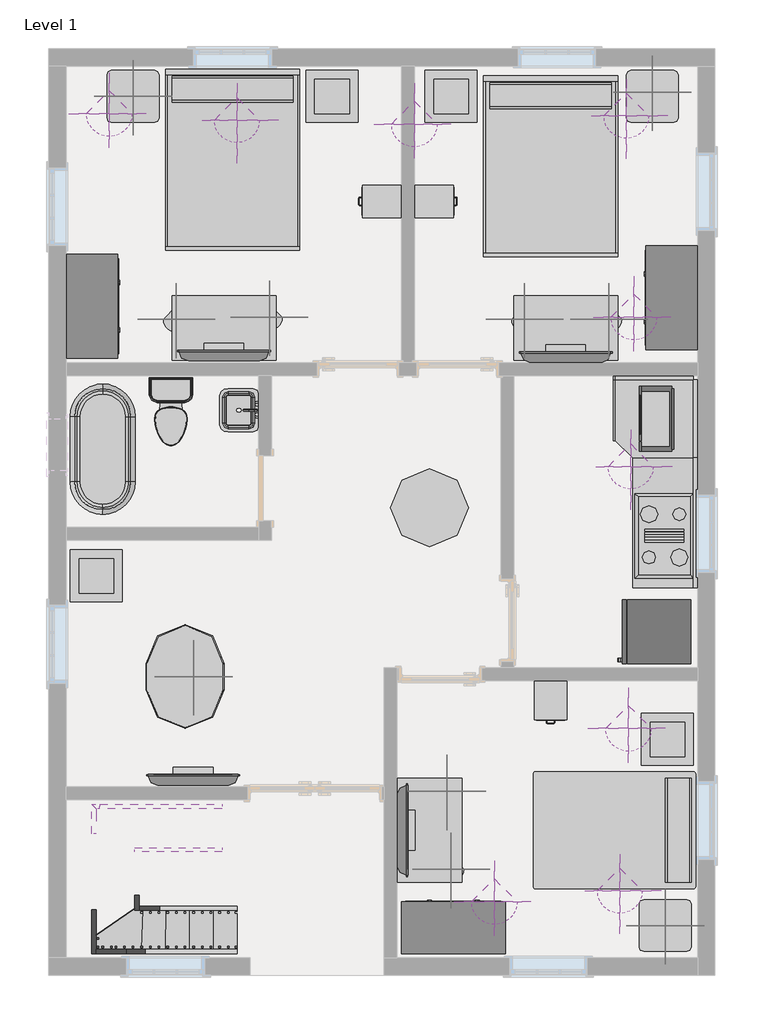
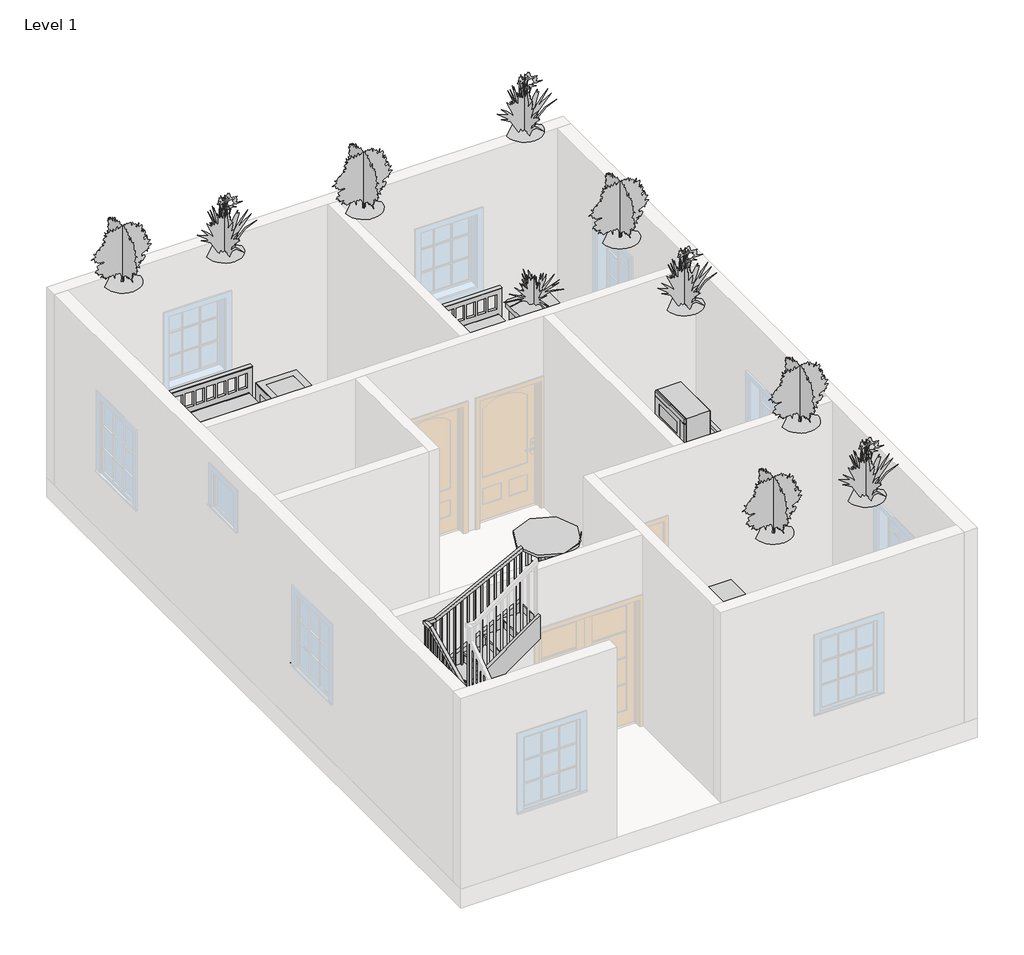
# One storey, part 2 of 2: 26 furniture elements, 19 geographic elements, 9 members, 4 flow terminals, 3 proxies, 1 railing, 1 stair flight.
"""IFC4 building model written with IfcOpenShell, lengths in millimetres."""

from ifc_helpers import new_model, si_unit, frame, origin, place, context, project, spatial, polyline, outline, extrude, faceted_brep, transform, mapped, element, save
from components import proxy_bb1e6e30, proxy_8a8d5ab2, proxy_a13a33b2, flow_terminal_accce45a, flow_terminal_62a433f7, toilet_domestic_3d_toilet_domestic_3d_f7549cf7, toilet_domestic_3d_toilet_domestic_3d_183bbd19, flow_terminal_b374fae2, furniture_35c09872, furniture_0253826f, furniture_bb55ed6b, furniture_9fa109b2, furniture_7a3aaa4f, furniture_b5c51a22, furniture_be1c6672, furniture_905aceb5, furniture_31d08a24, furniture_3f969c1c, furniture_f408c91c, rpc_plant_tropical_55f6ff97, rpc_plant_tropical_agave_1_5_93a2a214, rpc_plant_tropical_jungle_flame_3_9c4808c2, stair_flight_132ddc74

model = new_model("IFC4")

# Units and contexts
model_context = context("Model", 3, world=origin())
ifc_project = project(units=[si_unit("LENGTHUNIT", "METRE", prefix="MILLI")], contexts=[model_context])

# Site, building, storey
site = spatial("IfcSite", under=ifc_project)
building = spatial("IfcBuilding", under=site)
storey = spatial("IfcBuildingStorey", under=building, Name="Level 1", Elevation=0.0)

# Proxies
placement = place(None, origin())
proxy_shape = proxy_bb1e6e30(model_context)
element("IfcBuildingElementProxy", 1, Name="Cook Top-4 Unit : 36\" x 20\"", ObjectType="Cook Top-4 Unit : 36\" x 20\"", at=placement, inside=storey, context=model_context, shape_type="MappedRepresentation", body=[
    mapped(proxy_shape, transform((-5830.7047602, 8433.499435, 0.0), x_axis=(0.0, 1.0000000000000002, 0.0), y_axis=(-1.0000000000000002, 0.0, 0.0), z_axis=(0.0, 0.0, 1.0))),
])
proxy_2_shape = proxy_8a8d5ab2(model_context)
element("IfcBuildingElementProxy", 2, Name="Microwave : 30\" x 16\" x 18\"", ObjectType="Microwave : 30\" x 16\" x 18\"", at=placement, inside=storey, context=model_context, shape_type="MappedRepresentation", body=[
    mapped(proxy_2_shape, transform((-5566.5242544, 10305.3923123, 0.0), x_axis=(0.0, -1.0000000000000004, 0.0), y_axis=(1.0000000000000004, 0.0, 0.0), z_axis=(0.0, 0.0, 1.0))),
])
proxy_3_shape = proxy_a13a33b2(model_context)
element("IfcBuildingElementProxy", 3, Name="Refrigerator : 30\" x 32\" RH", ObjectType="Refrigerator : 30\" x 32\" RH", at=placement, inside=storey, context=model_context, shape_type="MappedRepresentation", body=[
    mapped(proxy_3_shape, transform((-5905.3172602, 7308.3504635, 0.0), x_axis=(0.0, -1.0000000000000007, 0.0), y_axis=(1.0000000000000007, 0.0, 0.0), z_axis=(0.0, 0.0, 1.0))),
])

# Flow terminals
flow_terminal_shape = flow_terminal_accce45a(model_context)
element("IfcFlowTerminal", 4, ObjectType="Floor Drain - Round : 5\" Strainer - 2\" Drain", at=placement, inside=storey, context=model_context, shape_type="MappedRepresentation", body=[
    mapped(flow_terminal_shape, transform((-11812.4047602, 8865.299435, 0.0), x_axis=(1.0, 0.0, 0.0), y_axis=(0.0, 1.0, 0.0), z_axis=(0.0, 0.0, 1.0))),
])
flow_terminal_2_shape = flow_terminal_62a433f7(model_context)
element("IfcFlowTerminal", 5, ObjectType="Sink Vanity-Square : 20\" x 18\"", at=placement, inside=storey, context=model_context, shape_type="MappedRepresentation", body=[
    mapped(flow_terminal_2_shape, transform((-10773.3501613, 9922.3886756, 0.0), x_axis=(0.0, -1.0000000000000002, 0.0), y_axis=(1.0000000000000002, 0.0, 0.0), z_axis=(0.0, 0.0, 1.0))),
])
toilet_domestic_3d_toilet_domestic_3d_shape = toilet_domestic_3d_toilet_domestic_3d_f7549cf7(model_context)
toilet_domestic_3d_toilet_domestic_3d_2_shape = toilet_domestic_3d_toilet_domestic_3d_183bbd19(model_context)
element("IfcFlowTerminal", 6, ObjectType="Toilet-Domestic-3D : Toilet-Domestic-3D", at=placement, inside=storey, context=model_context, shape_type="MappedRepresentation", body=[
    mapped(toilet_domestic_3d_toilet_domestic_3d_shape, transform((-11621.9047602, 9793.0034076, 0.0), x_axis=(1.0, 0.0, 0.0), y_axis=(0.0, 1.0, 0.0), z_axis=(0.0, 0.0, 1.0))),
    mapped(toilet_domestic_3d_toilet_domestic_3d_2_shape, transform((-11621.9047602, 9793.0034076, 0.0), x_axis=(1.0, 0.0, 0.0), y_axis=(0.0, 1.0, 0.0), z_axis=(0.0, 0.0, 1.0))),
])
flow_terminal_3_shape = flow_terminal_b374fae2(model_context)
element("IfcFlowTerminal", 7, ObjectType="Tub-Free Standing-3D : 30\" x 60\"", at=placement, inside=storey, context=model_context, shape_type="MappedRepresentation", body=[
    mapped(flow_terminal_3_shape, transform((-12422.0047602, 9449.499435, 0.0), x_axis=(1.0, 0.0, 0.0), y_axis=(0.0, 1.0, 0.0), z_axis=(0.0, 0.0, 1.0))),
])

# Furniture
furniture_shape = furniture_35c09872(model_context)
element("IfcFurniture", 8, ObjectType="Bed-Shaker : Queen 62\" x 83\"", at=placement, inside=storey, context=model_context, shape_type="MappedRepresentation", body=[
    mapped(furniture_shape, transform((-10878.9547602, 13894.499435, 0.0), x_axis=(1.0, 0.0, 0.0), y_axis=(0.0, 1.0, 0.0), z_axis=(0.0, 0.0, 1.0))),
])
element("IfcFurniture", 9, ObjectType="Bed-Shaker : Queen 62\" x 83\"", at=placement, inside=storey, context=model_context, shape_type="MappedRepresentation", body=[
    mapped(furniture_shape, transform((-7145.1547602, 13818.299435, 0.0), x_axis=(1.0, 0.0, 0.0), y_axis=(0.0, 1.0, 0.0), z_axis=(0.0, 0.0, 1.0))),
])
furniture_2_shape = furniture_0253826f(model_context)
element("IfcFurniture", 10, ObjectType="Bed-Standard.0001 : Double 54\" x 75\"", at=placement, inside=storey, context=model_context, shape_type="MappedRepresentation", body=[
    mapped(furniture_2_shape, transform((-6369.3096782, 5250.5879596, 0.0), x_axis=(0.0, -1.0000000000000002, 0.0), y_axis=(1.0000000000000002, 0.0, 0.0), z_axis=(0.0, 0.0, 1.0))),
])
furniture_3_shape = furniture_bb55ed6b(model_context)
element("IfcFurniture", 11, ObjectType="Cabinet-File 2 Drawer : 15\" x 18\"", at=placement, inside=storey, context=model_context, shape_type="MappedRepresentation", body=[
    mapped(furniture_3_shape, transform((-9003.2704601, 12229.9029879, 0.0), x_axis=(0.0, -1.0000000000000002, 0.0), y_axis=(1.0000000000000002, 0.0, 0.0), z_axis=(0.0, 0.0, 1.0))),
])
element("IfcFurniture", 12, ObjectType="Cabinet-File 2 Drawer : 15\" x 18\"", at=placement, inside=storey, context=model_context, shape_type="MappedRepresentation", body=[
    mapped(furniture_3_shape, transform((-8677.9390603, 12485.695882, 0.0), x_axis=(0.0, 1.0, 0.0), y_axis=(-1.0, 0.0, 0.0), z_axis=(0.0, 0.0, 1.0))),
])
element("IfcFurniture", 13, ObjectType="Cabinet-File 2 Drawer : 15\" x 18\"", at=placement, inside=storey, context=model_context, shape_type="MappedRepresentation", body=[
    mapped(furniture_3_shape, transform((-7036.2699762, 6645.2337351, 0.0), x_axis=(1.0, 0.0, 0.0), y_axis=(0.0, 1.0, 0.0), z_axis=(0.0, 0.0, 1.0))),
])
furniture_4_shape = furniture_9fa109b2(model_context)
element("IfcFurniture", 14, ObjectType="Dresser : 48\" x 72\" x 24\"", at=placement, inside=storey, context=model_context, shape_type="MappedRepresentation", body=[
    mapped(furniture_4_shape, transform((-12912.1677143, 11395.0926948, 0.0), x_axis=(0.0, 1.0, 0.0), y_axis=(-1.0, 0.0, 0.0), z_axis=(0.0, 0.0, 1.0))),
])
element("IfcFurniture", 15, ObjectType="Dresser : 48\" x 72\" x 24\"", at=placement, inside=storey, context=model_context, shape_type="MappedRepresentation", body=[
    mapped(furniture_4_shape, transform((-5378.6418061, 10958.3061751, 0.0), x_axis=(0.0, -1.0000000000000004, 0.0), y_axis=(1.0000000000000004, 0.0, 0.0), z_axis=(0.0, 0.0, 1.0))),
])
element("IfcFurniture", 16, ObjectType="Dresser : 48\" x 72\" x 24\"", at=placement, inside=storey, context=model_context, shape_type="MappedRepresentation", body=[
    mapped(furniture_4_shape, transform((-8576.3980201, 3472.9364809, 0.0), x_axis=(-1.0000000000000004, 0.0, 0.0), y_axis=(0.0, -1.0000000000000004, 0.0), z_axis=(0.0, 0.0, 1.0))),
])
furniture_5_shape = furniture_7a3aaa4f(model_context)
element("IfcFurniture", 17, ObjectType="TV - Flat Screen : 42\"", at=placement, inside=storey, context=model_context, shape_type="MappedRepresentation", body=[
    mapped(furniture_5_shape, transform((-11003.5492744, 10543.0880586, 1041.4), x_axis=(-1.0000000000000004, 0.0, 0.0), y_axis=(0.0, -1.0000000000000004, 0.0), z_axis=(0.0, 0.0, 1.0))),
])
element("IfcFurniture", 18, ObjectType="TV - Flat Screen : 42\"", at=placement, inside=storey, context=model_context, shape_type="MappedRepresentation", body=[
    mapped(furniture_5_shape, transform((-6990.3492744, 10524.0380586, 1041.4), x_axis=(-1.0000000000000004, 0.0, 0.0), y_axis=(0.0, -1.0000000000000004, 0.0), z_axis=(0.0, 0.0, 1.0))),
])
element("IfcFurniture", 19, ObjectType="TV - Flat Screen : 42\"", at=placement, inside=storey, context=model_context, shape_type="MappedRepresentation", body=[
    mapped(furniture_5_shape, transform((-8909.0661366, 4983.0439491, 1041.4), x_axis=(0.0, 1.0000000000000002, 0.0), y_axis=(-1.0000000000000002, 0.0, 0.0), z_axis=(0.0, 0.0, 1.0))),
])
element("IfcFurniture", 20, ObjectType="TV - Flat Screen : 42\"", at=placement, inside=storey, context=model_context, shape_type="MappedRepresentation", body=[
    mapped(furniture_5_shape, transform((-11365.4992744, 5564.6880586, 990.6), x_axis=(-1.0, 0.0, 0.0), y_axis=(0.0, -1.0, 0.0), z_axis=(0.0, 0.0, 1.0))),
])
furniture_6_shape = furniture_b5c51a22(model_context)
element("IfcFurniture", 21, ObjectType="Table-Coffee : 24\" x 24\" x 24\"", at=placement, inside=storey, context=model_context, shape_type="MappedRepresentation", body=[
    mapped(furniture_6_shape, transform((-9747.8705269, 13494.4883572, 0.0), x_axis=(1.0, 0.0, 0.0), y_axis=(0.0, 1.0, 0.0), z_axis=(0.0, 0.0, 1.0))),
])
element("IfcFurniture", 22, ObjectType="Table-Coffee : 24\" x 24\" x 24\"", at=placement, inside=storey, context=model_context, shape_type="MappedRepresentation", body=[
    mapped(furniture_6_shape, transform((-8350.8705269, 13494.4883572, 0.0), x_axis=(1.0, 0.0, 0.0), y_axis=(0.0, 1.0, 0.0), z_axis=(0.0, 0.0, 1.0))),
])
element("IfcFurniture", 23, ObjectType="Table-Coffee : 24\" x 24\" x 24\"", at=placement, inside=storey, context=model_context, shape_type="MappedRepresentation", body=[
    mapped(furniture_6_shape, transform((-12516.4705269, 7868.3883572, 0.0), x_axis=(1.0, 0.0, 0.0), y_axis=(0.0, 1.0, 0.0), z_axis=(0.0, 0.0, 1.0))),
])
element("IfcFurniture", 24, ObjectType="Table-Coffee : 24\" x 24\" x 24\"", at=placement, inside=storey, context=model_context, shape_type="MappedRepresentation", body=[
    mapped(furniture_6_shape, transform((-5810.8705269, 5950.6883572, 0.0), x_axis=(1.0, 0.0, 0.0), y_axis=(0.0, 1.0, 0.0), z_axis=(0.0, 0.0, 1.0))),
])
furniture_7_shape = furniture_be1c6672(model_context)
element("IfcFurniture", 25, ObjectType="Table-Dining Oval : 36\" x 48\"", at=placement, inside=storey, context=model_context, shape_type="MappedRepresentation", body=[
    mapped(furniture_7_shape, transform((-11814.9031209, 7184.3191071, 0.0), x_axis=(0.0, 1.0000000000000002, 0.0), y_axis=(-1.0000000000000002, 0.0, 0.0), z_axis=(0.0, 0.0, 1.0))),
])
furniture_8_shape = furniture_905aceb5(model_context)
element("IfcFurniture", 26, ObjectType="Table-Dining Round w Chairs : 36\" Diameter", at=placement, inside=storey, context=model_context, shape_type="MappedRepresentation", body=[
    mapped(furniture_8_shape, transform((-8690.2867274, 8948.5781235, 0.0), x_axis=(1.0, 0.0, 0.0), y_axis=(0.0, 1.0, 0.0), z_axis=(0.0, 0.0, 1.0))),
])
furniture_9_shape = furniture_31d08a24(model_context)
element("IfcFurniture", 27, ObjectType="Table-End : 24\" x 24\"", at=placement, inside=storey, context=model_context, shape_type="MappedRepresentation", body=[
    mapped(furniture_9_shape, transform((-12374.9383905, 13437.299435, 0.0), x_axis=(1.0, 0.0, 0.0), y_axis=(0.0, 1.0, 0.0), z_axis=(0.0, 0.0, 1.0))),
])
element("IfcFurniture", 28, ObjectType="Table-End : 24\" x 24\"", at=placement, inside=storey, context=model_context, shape_type="MappedRepresentation", body=[
    mapped(furniture_9_shape, transform((-6278.9383905, 13437.299435, 0.0), x_axis=(1.0, 0.0, 0.0), y_axis=(0.0, 1.0, 0.0), z_axis=(0.0, 0.0, 1.0))),
])
element("IfcFurniture", 29, ObjectType="Table-End : 24\" x 24\"", at=placement, inside=storey, context=model_context, shape_type="MappedRepresentation", body=[
    mapped(furniture_9_shape, transform((-6126.5383905, 3709.099435, 0.0), x_axis=(1.0, 0.0, 0.0), y_axis=(0.0, 1.0, 0.0), z_axis=(0.0, 0.0, 1.0))),
])
furniture_10_shape = furniture_3f969c1c(model_context)
element("IfcFurniture", 30, ObjectType="Table-Rectangular : 72\" x 30\"", at=placement, inside=storey, context=model_context, shape_type="MappedRepresentation", body=[
    mapped(furniture_10_shape, transform((-10999.6047602, 10871.899435, 0.0), x_axis=(1.0, 0.0, 0.0), y_axis=(0.0, 1.0, 0.0), z_axis=(0.0, 0.0, 1.0))),
])
element("IfcFurniture", 31, ObjectType="Table-Rectangular : 72\" x 30\"", at=placement, inside=storey, context=model_context, shape_type="MappedRepresentation", body=[
    mapped(furniture_10_shape, transform((-6986.4047602, 10871.899435, 0.0), x_axis=(1.0, 0.0, 0.0), y_axis=(0.0, 1.0, 0.0), z_axis=(0.0, 0.0, 1.0))),
])
element("IfcFurniture", 32, ObjectType="Table-Rectangular : 72\" x 30\"", at=placement, inside=storey, context=model_context, shape_type="MappedRepresentation", body=[
    mapped(furniture_10_shape, transform((-8586.6047602, 4979.099435, 0.0), x_axis=(0.0, 1.0000000000000002, 0.0), y_axis=(-1.0000000000000002, 0.0, 0.0), z_axis=(0.0, 0.0, 1.0))),
])
furniture_11_shape = furniture_f408c91c(model_context)
element("IfcFurniture", 33, ObjectType="Work Station Cubicle : 96\" x 96\"", at=placement, inside=storey, context=model_context, shape_type="MappedRepresentation", body=[
    mapped(furniture_11_shape, transform((-4941.9817526, 10181.3676828, 0.0), x_axis=(0.0, -1.0000000000000004, 0.0), y_axis=(1.0000000000000004, 0.0, 0.0), z_axis=(0.0, 0.0, 1.0))),
])

# Geographic elements
rpc_plant_tropical_shape = rpc_plant_tropical_55f6ff97(model_context)
element("IfcGeographicElement", 34, ObjectType="RPC Plant - Tropical", at=placement, inside=storey, context=model_context, shape_type="MappedRepresentation", body=[
    mapped(rpc_plant_tropical_shape, transform((-6275.2047602, 13361.099435, 3657.6), x_axis=(1.0, 0.0, 0.0), y_axis=(0.0, 1.0, 0.0), z_axis=(0.0, 0.0, 1.0))),
])
element("IfcGeographicElement", 35, ObjectType="RPC Plant - Tropical", at=placement, inside=storey, context=model_context, shape_type="MappedRepresentation", body=[
    mapped(rpc_plant_tropical_shape, transform((-10847.2047602, 13310.299435, 3352.8), x_axis=(1.0, 0.0, 0.0), y_axis=(0.0, 1.0, 0.0), z_axis=(0.0, 0.0, 1.0))),
])
element("IfcGeographicElement", 36, ObjectType="RPC Plant - Tropical", at=placement, inside=storey, context=model_context, shape_type="MappedRepresentation", body=[
    mapped(rpc_plant_tropical_shape, transform((-6351.4047602, 4267.899435, 3352.8), x_axis=(1.0, 0.0, 0.0), y_axis=(0.0, 1.0, 0.0), z_axis=(0.0, 0.0, 1.0))),
])
element("IfcGeographicElement", 37, ObjectType="RPC Plant - Tropical", at=placement, inside=storey, context=model_context, shape_type="MappedRepresentation", body=[
    mapped(rpc_plant_tropical_shape, transform((-6224.4047602, 9246.299435, 3352.8), x_axis=(1.0, 0.0, 0.0), y_axis=(0.0, 1.0, 0.0), z_axis=(0.0, 0.0, 1.0))),
])
rpc_plant_tropical_agave_1_5_shape = rpc_plant_tropical_agave_1_5_93a2a214(model_context)
element("IfcGeographicElement", 38, ObjectType="RPC Plant - Tropical : Agave - 1.5'", at=placement, inside=storey, context=model_context, shape_type="MappedRepresentation", body=[
    mapped(rpc_plant_tropical_agave_1_5_shape, transform((-12066.4047602, 13589.699435, 609.6), x_axis=(1.0, 0.0, 0.0), y_axis=(0.0, 1.0, 0.0), z_axis=(0.0, 0.0, 1.0))),
])
element("IfcGeographicElement", 39, ObjectType="RPC Plant - Tropical : Agave - 1.5'", at=placement, inside=storey, context=model_context, shape_type="MappedRepresentation", body=[
    mapped(rpc_plant_tropical_agave_1_5_shape, transform((-11558.4047602, 10973.499435, 660.4), x_axis=(1.0, 0.0, 0.0), y_axis=(0.0, 1.0, 0.0), z_axis=(0.0, 0.0, 1.0))),
])
element("IfcGeographicElement", 40, ObjectType="RPC Plant - Tropical : Agave - 1.5'", at=placement, inside=storey, context=model_context, shape_type="MappedRepresentation", body=[
    mapped(rpc_plant_tropical_agave_1_5_shape, transform((-10466.2047602, 10998.899435, 660.4), x_axis=(1.0, 0.0, 0.0), y_axis=(0.0, 1.0, 0.0), z_axis=(0.0, 0.0, 1.0))),
])
element("IfcGeographicElement", 41, ObjectType="RPC Plant - Tropical : Agave - 1.5'", at=placement, inside=storey, context=model_context, shape_type="MappedRepresentation", body=[
    mapped(rpc_plant_tropical_agave_1_5_shape, transform((-5970.4047602, 13640.499435, 609.6), x_axis=(1.0, 0.0, 0.0), y_axis=(0.0, 1.0, 0.0), z_axis=(0.0, 0.0, 1.0))),
])
element("IfcGeographicElement", 42, ObjectType="RPC Plant - Tropical : Agave - 1.5'", at=placement, inside=storey, context=model_context, shape_type="MappedRepresentation", body=[
    mapped(rpc_plant_tropical_agave_1_5_shape, transform((-7469.0047602, 10973.499435, 660.4), x_axis=(1.0, 0.0, 0.0), y_axis=(0.0, 1.0, 0.0), z_axis=(0.0, 0.0, 1.0))),
])
element("IfcGeographicElement", 43, ObjectType="RPC Plant - Tropical : Agave - 1.5'", at=placement, inside=storey, context=model_context, shape_type="MappedRepresentation", body=[
    mapped(rpc_plant_tropical_agave_1_5_shape, transform((-6478.4047602, 10973.499435, 660.4), x_axis=(1.0, 0.0, 0.0), y_axis=(0.0, 1.0, 0.0), z_axis=(0.0, 0.0, 1.0))),
])
element("IfcGeographicElement", 44, ObjectType="RPC Plant - Tropical : Agave - 1.5'", at=placement, inside=storey, context=model_context, shape_type="MappedRepresentation", body=[
    mapped(rpc_plant_tropical_agave_1_5_shape, transform((-11355.2047602, 6782.499435, 736.6), x_axis=(1.0, 0.0, 0.0), y_axis=(0.0, 1.0, 0.0), z_axis=(0.0, 0.0, 1.0))),
])
element("IfcGeographicElement", 45, ObjectType="RPC Plant - Tropical : Agave - 1.5'", at=placement, inside=storey, context=model_context, shape_type="MappedRepresentation", body=[
    mapped(rpc_plant_tropical_agave_1_5_shape, transform((-5818.0047602, 3861.499435, 609.6), x_axis=(1.0, 0.0, 0.0), y_axis=(0.0, 1.0, 0.0), z_axis=(0.0, 0.0, 1.0))),
])
element("IfcGeographicElement", 46, ObjectType="RPC Plant - Tropical : Agave - 1.5'", at=placement, inside=storey, context=model_context, shape_type="MappedRepresentation", body=[
    mapped(rpc_plant_tropical_agave_1_5_shape, transform((-8383.4047602, 5436.299435, 660.4), x_axis=(1.0, 0.0, 0.0), y_axis=(0.0, 1.0, 0.0), z_axis=(0.0, 0.0, 1.0))),
])
element("IfcGeographicElement", 47, ObjectType="RPC Plant - Tropical : Agave - 1.5'", at=placement, inside=storey, context=model_context, shape_type="MappedRepresentation", body=[
    mapped(rpc_plant_tropical_agave_1_5_shape, transform((-8332.6047602, 4521.899435, 660.4), x_axis=(1.0, 0.0, 0.0), y_axis=(0.0, 1.0, 0.0), z_axis=(0.0, 0.0, 1.0))),
])
rpc_plant_tropical_jungle_flame_3_shape = rpc_plant_tropical_jungle_flame_3_9c4808c2(model_context)
element("IfcGeographicElement", 48, ObjectType="RPC Plant - Tropical : Jungle Flame - 3'", at=placement, inside=storey, context=model_context, shape_type="MappedRepresentation", body=[
    mapped(rpc_plant_tropical_jungle_flame_3_shape, transform((-8764.4047602, 13263.9821211, 3352.8), x_axis=(1.0, 0.0, 0.0), y_axis=(0.0, 1.0, 0.0), z_axis=(0.0, 0.0, 1.0))),
])
element("IfcGeographicElement", 49, ObjectType="RPC Plant - Tropical : Jungle Flame - 3'", at=placement, inside=storey, context=model_context, shape_type="MappedRepresentation", body=[
    mapped(rpc_plant_tropical_jungle_flame_3_shape, transform((-12345.8047602, 13386.499435, 3352.8), x_axis=(1.0, 0.0, 0.0), y_axis=(0.0, 1.0, 0.0), z_axis=(0.0, 0.0, 1.0))),
])
element("IfcGeographicElement", 50, ObjectType="RPC Plant - Tropical : Jungle Flame - 3'", at=placement, inside=storey, context=model_context, shape_type="MappedRepresentation", body=[
    mapped(rpc_plant_tropical_jungle_flame_3_shape, transform((-6186.3047602, 10998.899435, 3352.8), x_axis=(1.0, 0.0, 0.0), y_axis=(0.0, 1.0, 0.0), z_axis=(0.0, 0.0, 1.0))),
])
element("IfcGeographicElement", 51, ObjectType="RPC Plant - Tropical : Jungle Flame - 3'", at=placement, inside=storey, context=model_context, shape_type="MappedRepresentation", body=[
    mapped(rpc_plant_tropical_jungle_flame_3_shape, transform((-7824.6047602, 4140.899435, 3352.8), x_axis=(1.0, 0.0, 0.0), y_axis=(0.0, 1.0, 0.0), z_axis=(0.0, 0.0, 1.0))),
])
element("IfcGeographicElement", 52, ObjectType="RPC Plant - Tropical : Jungle Flame - 3'", at=placement, inside=storey, context=model_context, shape_type="MappedRepresentation", body=[
    mapped(rpc_plant_tropical_jungle_flame_3_shape, transform((-6249.8047602, 6172.899435, 3352.8), x_axis=(1.0, 0.0, 0.0), y_axis=(0.0, 1.0, 0.0), z_axis=(0.0, 0.0, 1.0))),
])

# Members
element("IfcMember", 53, ObjectType="Stringer - 2\" Width", at=placement, inside=storey, context=model_context, shape_type="SweptSolid", body=[
    extrude(outline(polyline([(196.4096939, -10847.2047602), (551.886059, -10847.2047602), (1331.4686735, -12146.2117977), (975.9923084, -12146.2117977), (196.4096939, -10847.2047602)])), frame((0.0, 3531.299435, 0.0), z_axis=(0.0, 1.0, 0.0), x_axis=(0.0, 0.0, 1.0)), (0.0, 0.0, 1.0), 50.8),
])
element("IfcMember", 54, ObjectType="Stringer - 2\" Width", at=placement, inside=storey, context=model_context, shape_type="SweptSolid", body=[
    extrude(outline(polyline([(-12146.2117977, 3582.099435), (-12146.2117977, 3531.299435), (-12501.9364521, 3531.299435), (-12501.9364521, 3582.099435), (-12146.2117977, 3582.099435)])), frame((0.0, 0.0, 975.9923084), z_axis=(0.0, 0.0, 1.0), x_axis=(1.0, 0.0, 0.0)), (0.0, 0.0, 1.0), 355.4763651),
])
element("IfcMember", 55, ObjectType="Stringer - 2\" Width", at=placement, inside=storey, context=model_context, shape_type="SweptSolid", body=[
    extrude(outline(polyline([(3531.299435, 1026.6686735), (3531.299435, 1306.8449342), (4939.7837414, 1989.5644288), (4939.7837414, 1634.0880637), (3686.6472991, 1026.6686735), (3531.299435, 1026.6686735)])), frame((-12552.7364521, 0.0, 0.0), z_axis=(1.0, 0.0, 0.0), x_axis=(0.0, 1.0, 0.0)), (0.0, 0.0, 1.0), 50.8),
])
element("IfcMember", 56, ObjectType="Stringer - 2\" Width", at=placement, inside=storey, context=model_context, shape_type="SweptSolid", body=[
    extrude(outline(polyline([(-12501.9364521, 4939.7837414), (-12552.7364521, 4939.7837414), (-12552.7364521, 5283.899435), (-12501.9364521, 5233.099435), (-12501.9364521, 4939.7837414)])), frame((0.0, 0.0, 1641.2436104), z_axis=(0.0, 0.0, 1.0), x_axis=(1.0, 0.0, 0.0)), (0.0, 0.0, 1.0), 338.7194522),
])
element("IfcMember", 57, ObjectType="Stringer - 2\" Width", at=placement, inside=storey, context=model_context, shape_type="SweptSolid", body=[
    extrude(outline(polyline([(-12501.9364521, 5233.099435), (-12552.7364521, 5283.899435), (-12456.259975, 5283.899435), (-12456.259975, 5233.099435), (-12501.9364521, 5233.099435)])), frame((0.0, 0.0, 1641.2436104), z_axis=(0.0, 0.0, 1.0), x_axis=(1.0, 0.0, 0.0)), (0.0, 0.0, 1.0), 338.7194522),
])
element("IfcMember", 58, ObjectType="Stringer - 2\" Width", at=placement, inside=storey, context=model_context, shape_type="SweptSolid", body=[
    extrude(outline(polyline([(144.118617, -10847.2047602), (525.298754, -10847.2047602), (1386.4765807, -11993.9364521), (1005.2964437, -11993.9364521), (144.118617, -10847.2047602)])), frame((0.0, 4039.299435, 0.0), z_axis=(0.0, 1.0, 0.0), x_axis=(0.0, 0.0, 1.0)), (0.0, 0.0, 1.0), 50.8),
])
element("IfcMember", 59, ObjectType="Stringer - 2\" Width", at=placement, inside=storey, context=model_context, shape_type="SweptSolid", body=[
    extrude(outline(polyline([(4039.299435, 1078.8769196), (4039.299435, 1449.5381091), (4725.099435, 1924.105074), (4725.099435, 1553.4438846), (4039.299435, 1078.8769196)])), frame((-12044.7364521, 0.0, 0.0), z_axis=(1.0, 0.0, 0.0), x_axis=(0.0, 1.0, 0.0)), (0.0, 0.0, 1.0), 50.8),
])
element("IfcMember", 60, ObjectType="Stringer - 2\" Width", at=placement, inside=storey, context=model_context, shape_type="SweptSolid", body=[
    extrude(outline(polyline([(2064.1743094, -12044.7364521), (1689.6875316, -12044.7364521), (2418.6253368, -11023.5532442), (2793.1121146, -11023.5532442), (2064.1743094, -12044.7364521)])), frame((0.0, 4725.099435, 0.0), z_axis=(0.0, 1.0, 0.0), x_axis=(0.0, 0.0, 1.0)), (0.0, 0.0, 1.0), 50.8),
])
element("IfcMember", 61, ObjectType="Stringer - 2\" Width", at=placement, inside=storey, context=model_context, shape_type="SweptSolid", body=[
    extrude(outline(polyline([(1979.9630626, -12456.259975), (1641.2436104, -12456.259975), (2377.4896582, -11023.5532442), (2716.2091104, -11023.5532442), (1979.9630626, -12456.259975)])), frame((0.0, 5233.099435, 0.0), z_axis=(0.0, 1.0, 0.0), x_axis=(0.0, 0.0, 1.0)), (0.0, 0.0, 1.0), 50.8),
])

# Railing
element("IfcRailing", 62, ObjectType="Handrail - Rectangular", at=placement, inside=storey, context=model_context, shape_type="SolidModel", body=[
    faceted_brep([(-10847.2047602, 3582.099435, 1424.0549635), (-10847.2047602, 3582.099435, 1364.8089026), (-10847.2047602, 3632.899435, 1364.8089026), (-10847.2047602, 3632.899435, 1424.0549635), (-12321.6316685, 3582.099435, 2308.9135908), (-12335.7052154, 3582.099435, 2258.1135908), (-12335.7052154, 3632.899435, 2258.1135908), (-12321.6316685, 3632.899435, 2308.9135908), (-12501.9364521, 3582.099435, 2308.9135908), (-12501.9364521, 3582.099435, 2258.1135908), (-12451.1364521, 3632.899435, 2258.1135908), (-12451.1364521, 3632.899435, 2308.9135908), (-12501.9364521, 3799.2890905, 2308.9135908), (-12501.9364521, 3810.9520103, 2258.1135908), (-12451.1364521, 3810.9520103, 2258.1135908), (-12451.1364521, 3799.2890905, 2308.9135908), (-12501.9364521, 5062.993335, 2921.4553984), (-12501.9364521, 5074.6562547, 2870.6553984), (-12451.1364521, 5074.6562547, 2870.6553984), (-12451.1364521, 5062.993335, 2921.4553984), (-12501.9364521, 5233.099435, 2921.4553984), (-12501.9364521, 5233.099435, 2870.6553984), (-12451.1364521, 5182.299435, 2870.6553984), (-12451.1364521, 5182.299435, 2921.4553984), (-12340.0431139, 5233.099435, 2921.4553984), (-12327.7542684, 5233.099435, 2870.6553984), (-12327.7542684, 5182.299435, 2870.6553984), (-12340.0431139, 5182.299435, 2921.4553984), (-11023.5532442, 5233.099435, 3597.9793811), (-11023.5532442, 5182.299435, 3597.9793811), (-11023.5532442, 5182.299435, 3540.8643316), (-11023.5532442, 5233.099435, 3540.8643316)], [[[0, 1, 2, 3]], [[1, 0, 4, 5]], [[2, 1, 5, 6]], [[3, 2, 6, 7]], [[0, 3, 7, 4]], [[5, 4, 8, 9]], [[6, 5, 9, 10]], [[7, 6, 10, 11]], [[4, 7, 11, 8]], [[9, 8, 12, 13]], [[10, 9, 13, 14]], [[11, 10, 14, 15]], [[8, 11, 15, 12]], [[13, 12, 16, 17]], [[14, 13, 17, 18]], [[15, 14, 18, 19]], [[12, 15, 19, 16]], [[17, 16, 20, 21]], [[18, 17, 21, 22]], [[19, 18, 22, 23]], [[16, 19, 23, 20]], [[21, 20, 24, 25]], [[22, 21, 25, 26]], [[23, 22, 26, 27]], [[20, 23, 27, 24]], [[28, 29, 30, 31]], [[25, 24, 28, 31]], [[26, 25, 31, 30]], [[27, 26, 30, 29]], [[24, 27, 29, 28]]]),
    extrude(outline(polyline([(3485.9738059, -11130.3681139), (2540.0, -11130.3681139), (2540.0, -11111.3181139), (3495.7633091, -11111.3181139), (3485.9738059, -11130.3681139)])), frame((0.0, 5198.174435, 0.0), z_axis=(0.0, 1.0, 0.0), x_axis=(0.0, 0.0, 1.0)), (0.0, 0.0, 1.0), 19.05),
    extrude(outline(polyline([(3433.7631218, -11231.9681139), (2540.0, -11231.9681139), (2540.0, -11212.9181139), (3443.5526251, -11212.9181139), (3433.7631218, -11231.9681139)])), frame((0.0, 5198.174435, 0.0), z_axis=(0.0, 1.0, 0.0), x_axis=(0.0, 0.0, 1.0)), (0.0, 0.0, 1.0), 19.05),
    extrude(outline(polyline([(3381.5524378, -11333.5681139), (2370.6666667, -11333.5681139), (2370.6666667, -11314.5181139), (3391.341941, -11314.5181139), (3381.5524378, -11333.5681139)])), frame((0.0, 5198.174435, 0.0), z_axis=(0.0, 1.0, 0.0), x_axis=(0.0, 0.0, 1.0)), (0.0, 0.0, 1.0), 19.05),
    extrude(outline(polyline([(3329.3417537, -11435.1681139), (2370.6666667, -11435.1681139), (2370.6666667, -11416.1181139), (3339.131257, -11416.1181139), (3329.3417537, -11435.1681139)])), frame((0.0, 5198.174435, 0.0), z_axis=(0.0, 1.0, 0.0), x_axis=(0.0, 0.0, 1.0)), (0.0, 0.0, 1.0), 19.05),
    extrude(outline(polyline([(3277.1310697, -11536.7681139), (2370.6666667, -11536.7681139), (2370.6666667, -11517.7181139), (3286.9205729, -11517.7181139), (3277.1310697, -11536.7681139)])), frame((0.0, 5198.174435, 0.0), z_axis=(0.0, 1.0, 0.0), x_axis=(0.0, 0.0, 1.0)), (0.0, 0.0, 1.0), 19.05),
    extrude(outline(polyline([(3224.9203856, -11638.3681139), (2201.3333333, -11638.3681139), (2201.3333333, -11619.3181139), (3234.7098889, -11619.3181139), (3224.9203856, -11638.3681139)])), frame((0.0, 5198.174435, 0.0), z_axis=(0.0, 1.0, 0.0), x_axis=(0.0, 0.0, 1.0)), (0.0, 0.0, 1.0), 19.05),
    extrude(outline(polyline([(3172.7097016, -11739.9681139), (2201.3333333, -11739.9681139), (2201.3333333, -11720.9181139), (3182.4992048, -11720.9181139), (3172.7097016, -11739.9681139)])), frame((0.0, 5198.174435, 0.0), z_axis=(0.0, 1.0, 0.0), x_axis=(0.0, 0.0, 1.0)), (0.0, 0.0, 1.0), 19.05),
    extrude(outline(polyline([(3120.4990175, -11841.5681139), (2201.3333333, -11841.5681139), (2201.3333333, -11822.5181139), (3130.2885208, -11822.5181139), (3120.4990175, -11841.5681139)])), frame((0.0, 5198.174435, 0.0), z_axis=(0.0, 1.0, 0.0), x_axis=(0.0, 0.0, 1.0)), (0.0, 0.0, 1.0), 19.05),
    extrude(outline(polyline([(3068.2883335, -11943.1681139), (2032.0, -11943.1681139), (2032.0, -11924.1181139), (3078.0778367, -11924.1181139), (3068.2883335, -11943.1681139)])), frame((0.0, 5198.174435, 0.0), z_axis=(0.0, 1.0, 0.0), x_axis=(0.0, 0.0, 1.0)), (0.0, 0.0, 1.0), 19.05),
    extrude(outline(polyline([(3016.0776494, -12044.7681139), (2032.0, -12044.7681139), (2032.0, -12025.7181139), (3025.8671527, -12025.7181139), (3016.0776494, -12044.7681139)])), frame((0.0, 5198.174435, 0.0), z_axis=(0.0, 1.0, 0.0), x_axis=(0.0, 0.0, 1.0)), (0.0, 0.0, 1.0), 19.05),
    extrude(outline(polyline([(2963.8669654, -12146.3681139), (2032.0, -12146.3681139), (2032.0, -12127.3181139), (2973.6564686, -12127.3181139), (2963.8669654, -12146.3681139)])), frame((0.0, 5198.174435, 0.0), z_axis=(0.0, 1.0, 0.0), x_axis=(0.0, 0.0, 1.0)), (0.0, 0.0, 1.0), 19.05),
    extrude(outline(polyline([(2911.6562813, -12247.9681139), (2032.0, -12247.9681139), (2032.0, -12228.9181139), (2921.4457846, -12228.9181139), (2911.6562813, -12247.9681139)])), frame((0.0, 5198.174435, 0.0), z_axis=(0.0, 1.0, 0.0), x_axis=(0.0, 0.0, 1.0)), (0.0, 0.0, 1.0), 19.05),
    extrude(outline(polyline([(-12384.4614521, 5217.224435), (-12365.4114521, 5217.224435), (-12365.4114521, 5198.174435), (-12384.4614521, 5198.174435), (-12384.4614521, 5217.224435)])), frame((0.0, 0.0, 1862.6666667), z_axis=(0.0, 0.0, 1.0), x_axis=(1.0, 0.0, 0.0)), (0.0, 0.0, 1.0), 1007.9887318),
    extrude(outline(polyline([(-12486.0614521, 5155.068335), (-12486.0614521, 5174.118335), (-12467.0114521, 5174.118335), (-12467.0114521, 5155.068335), (-12486.0614521, 5155.068335)])), frame((0.0, 0.0, 1862.6666667), z_axis=(0.0, 0.0, 1.0), x_axis=(1.0, 0.0, 0.0)), (0.0, 0.0, 1.0), 1007.9887318),
    extrude(outline(polyline([(5028.0140905, 2848.0470423), (5028.0140905, 1862.6666667), (5008.9640905, 1862.6666667), (5008.9640905, 2838.8131401), (5028.0140905, 2848.0470423)])), frame((-12486.0614521, 0.0, 0.0), z_axis=(1.0, 0.0, 0.0), x_axis=(0.0, 1.0, 0.0)), (0.0, 0.0, 1.0), 19.05),
    extrude(outline(polyline([(4926.4140905, 2798.7995638), (4926.4140905, 1862.6666667), (4907.3640905, 1862.6666667), (4907.3640905, 2789.5656616), (4926.4140905, 2798.7995638)])), frame((-12486.0614521, 0.0, 0.0), z_axis=(1.0, 0.0, 0.0), x_axis=(0.0, 1.0, 0.0)), (0.0, 0.0, 1.0), 19.05),
    extrude(outline(polyline([(4824.8140905, 2749.5520852), (4824.8140905, 1862.6666667), (4805.7640905, 1862.6666667), (4805.7640905, 2740.318183), (4824.8140905, 2749.5520852)])), frame((-12486.0614521, 0.0, 0.0), z_axis=(1.0, 0.0, 0.0), x_axis=(0.0, 1.0, 0.0)), (0.0, 0.0, 1.0), 19.05),
    extrude(outline(polyline([(4723.2140905, 2700.2857742), (4723.2140905, 1693.3333333), (4704.1640905, 1693.3333333), (4704.1640905, 2691.051872), (4723.2140905, 2700.2857742)])), frame((-12486.0614521, 0.0, 0.0), z_axis=(1.0, 0.0, 0.0), x_axis=(0.0, 1.0, 0.0)), (0.0, 0.0, 1.0), 19.05),
    extrude(outline(polyline([(4621.6140905, 2651.0571282), (4621.6140905, 1693.3333333), (4602.5640905, 1693.3333333), (4602.5640905, 2641.8232259), (4621.6140905, 2651.0571282)])), frame((-12486.0614521, 0.0, 0.0), z_axis=(1.0, 0.0, 0.0), x_axis=(0.0, 1.0, 0.0)), (0.0, 0.0, 1.0), 19.05),
    extrude(outline(polyline([(4520.0140905, 2601.8096496), (4520.0140905, 1693.3333333), (4500.9640905, 1693.3333333), (4500.9640905, 2592.5757474), (4520.0140905, 2601.8096496)])), frame((-12486.0614521, 0.0, 0.0), z_axis=(1.0, 0.0, 0.0), x_axis=(0.0, 1.0, 0.0)), (0.0, 0.0, 1.0), 19.05),
    extrude(outline(polyline([(4418.4140905, 2552.5621711), (4418.4140905, 1524.0), (4399.3640905, 1524.0), (4399.3640905, 2543.3282689), (4418.4140905, 2552.5621711)])), frame((-12486.0614521, 0.0, 0.0), z_axis=(1.0, 0.0, 0.0), x_axis=(0.0, 1.0, 0.0)), (0.0, 0.0, 1.0), 19.05),
    extrude(outline(polyline([(4316.8140905, 2503.3146926), (4316.8140905, 1524.0), (4297.7640905, 1524.0), (4297.7640905, 2494.0807903), (4316.8140905, 2503.3146926)])), frame((-12486.0614521, 0.0, 0.0), z_axis=(1.0, 0.0, 0.0), x_axis=(0.0, 1.0, 0.0)), (0.0, 0.0, 1.0), 19.05),
    extrude(outline(polyline([(4215.2140905, 2454.067214), (4215.2140905, 1524.0), (4196.1640905, 1524.0), (4196.1640905, 2444.8333118), (4215.2140905, 2454.067214)])), frame((-12486.0614521, 0.0, 0.0), z_axis=(1.0, 0.0, 0.0), x_axis=(0.0, 1.0, 0.0)), (0.0, 0.0, 1.0), 19.05),
    extrude(outline(polyline([(4113.6140905, 2404.8197355), (4113.6140905, 1354.6666667), (4094.5640905, 1354.6666667), (4094.5640905, 2395.5858333), (4113.6140905, 2404.8197355)])), frame((-12486.0614521, 0.0, 0.0), z_axis=(1.0, 0.0, 0.0), x_axis=(0.0, 1.0, 0.0)), (0.0, 0.0, 1.0), 19.05),
    extrude(outline(polyline([(4012.0140905, 2355.5722569), (4012.0140905, 1354.6666667), (3992.9640905, 1354.6666667), (3992.9640905, 2346.3383547), (4012.0140905, 2355.5722569)])), frame((-12486.0614521, 0.0, 0.0), z_axis=(1.0, 0.0, 0.0), x_axis=(0.0, 1.0, 0.0)), (0.0, 0.0, 1.0), 19.05),
    extrude(outline(polyline([(3910.4140905, 2306.3247784), (3910.4140905, 1354.6666667), (3891.3640905, 1354.6666667), (3891.3640905, 2297.0908762), (3910.4140905, 2306.3247784)])), frame((-12486.0614521, 0.0, 0.0), z_axis=(1.0, 0.0, 0.0), x_axis=(0.0, 1.0, 0.0)), (0.0, 0.0, 1.0), 19.05),
    extrude(outline(polyline([(-12486.0614521, 3699.574435), (-12486.0614521, 3718.624435), (-12467.0114521, 3718.624435), (-12467.0114521, 3699.574435), (-12486.0614521, 3699.574435)])), frame((0.0, 0.0, 1185.3333333), z_axis=(0.0, 0.0, 1.0), x_axis=(1.0, 0.0, 0.0)), (0.0, 0.0, 1.0), 1072.7802574),
    extrude(outline(polyline([(-12413.7066685, 3597.974435), (-12432.7566685, 3597.974435), (-12432.7566685, 3617.024435), (-12413.7066685, 3617.024435), (-12413.7066685, 3597.974435)])), frame((0.0, 0.0, 1185.3333333), z_axis=(0.0, 0.0, 1.0), x_axis=(1.0, 0.0, 0.0)), (0.0, 0.0, 1.0), 1072.7802574),
    extrude(outline(polyline([(2224.1605482, -12279.1297602), (1185.3333333, -12279.1297602), (1185.3333333, -12260.0797602), (2212.7279321, -12260.0797602), (2224.1605482, -12279.1297602)])), frame((0.0, 3597.974435, 0.0), z_axis=(0.0, 1.0, 0.0), x_axis=(0.0, 0.0, 1.0)), (0.0, 0.0, 1.0), 19.05),
    extrude(outline(polyline([(2163.1865955, -12177.5297602), (1185.3333333, -12177.5297602), (1185.3333333, -12158.4797602), (2151.7539794, -12158.4797602), (2163.1865955, -12177.5297602)])), frame((0.0, 3597.974435, 0.0), z_axis=(0.0, 1.0, 0.0), x_axis=(0.0, 0.0, 1.0)), (0.0, 0.0, 1.0), 19.05),
    extrude(outline(polyline([(2102.2126428, -12075.9297602), (1185.3333333, -12075.9297602), (1185.3333333, -12056.8797602), (2090.7800267, -12056.8797602), (2102.2126428, -12075.9297602)])), frame((0.0, 3597.974435, 0.0), z_axis=(0.0, 1.0, 0.0), x_axis=(0.0, 0.0, 1.0)), (0.0, 0.0, 1.0), 19.05),
    extrude(outline(polyline([(2041.2386902, -11974.3297602), (1016.0, -11974.3297602), (1016.0, -11955.2797602), (2029.806074, -11955.2797602), (2041.2386902, -11974.3297602)])), frame((0.0, 3597.974435, 0.0), z_axis=(0.0, 1.0, 0.0), x_axis=(0.0, 0.0, 1.0)), (0.0, 0.0, 1.0), 19.05),
    extrude(outline(polyline([(1980.2647375, -11872.7297602), (1016.0, -11872.7297602), (1016.0, -11853.6797602), (1968.8321214, -11853.6797602), (1980.2647375, -11872.7297602)])), frame((0.0, 3597.974435, 0.0), z_axis=(0.0, 1.0, 0.0), x_axis=(0.0, 0.0, 1.0)), (0.0, 0.0, 1.0), 19.05),
    extrude(outline(polyline([(1919.2907848, -11771.1297602), (1016.0, -11771.1297602), (1016.0, -11752.0797602), (1907.8581687, -11752.0797602), (1919.2907848, -11771.1297602)])), frame((0.0, 3597.974435, 0.0), z_axis=(0.0, 1.0, 0.0), x_axis=(0.0, 0.0, 1.0)), (0.0, 0.0, 1.0), 19.05),
    extrude(outline(polyline([(1858.3168321, -11669.5297602), (846.6666667, -11669.5297602), (846.6666667, -11650.4797602), (1846.884216, -11650.4797602), (1858.3168321, -11669.5297602)])), frame((0.0, 3597.974435, 0.0), z_axis=(0.0, 1.0, 0.0), x_axis=(0.0, 0.0, 1.0)), (0.0, 0.0, 1.0), 19.05),
    extrude(outline(polyline([(1797.3428794, -11567.9297602), (846.6666667, -11567.9297602), (846.6666667, -11548.8797602), (1785.9102633, -11548.8797602), (1797.3428794, -11567.9297602)])), frame((0.0, 3597.974435, 0.0), z_axis=(0.0, 1.0, 0.0), x_axis=(0.0, 0.0, 1.0)), (0.0, 0.0, 1.0), 19.05),
    extrude(outline(polyline([(1736.3689268, -11466.3297602), (846.6666667, -11466.3297602), (846.6666667, -11447.2797602), (1724.9363106, -11447.2797602), (1736.3689268, -11466.3297602)])), frame((0.0, 3597.974435, 0.0), z_axis=(0.0, 1.0, 0.0), x_axis=(0.0, 0.0, 1.0)), (0.0, 0.0, 1.0), 19.05),
    extrude(outline(polyline([(1675.3949741, -11364.7297602), (677.3333333, -11364.7297602), (677.3333333, -11345.6797602), (1663.9623579, -11345.6797602), (1675.3949741, -11364.7297602)])), frame((0.0, 3597.974435, 0.0), z_axis=(0.0, 1.0, 0.0), x_axis=(0.0, 0.0, 1.0)), (0.0, 0.0, 1.0), 19.05),
    extrude(outline(polyline([(1614.4210214, -11263.1297602), (677.3333333, -11263.1297602), (677.3333333, -11244.0797602), (1602.9884053, -11244.0797602), (1614.4210214, -11263.1297602)])), frame((0.0, 3597.974435, 0.0), z_axis=(0.0, 1.0, 0.0), x_axis=(0.0, 0.0, 1.0)), (0.0, 0.0, 1.0), 19.05),
    extrude(outline(polyline([(1553.4470687, -11161.5297602), (677.3333333, -11161.5297602), (677.3333333, -11142.4797602), (1542.0144526, -11142.4797602), (1553.4470687, -11161.5297602)])), frame((0.0, 3597.974435, 0.0), z_axis=(0.0, 1.0, 0.0), x_axis=(0.0, 0.0, 1.0)), (0.0, 0.0, 1.0), 19.05),
    extrude(outline(polyline([(1492.473116, -11059.9297602), (508.0, -11059.9297602), (508.0, -11040.8797602), (1481.0404999, -11040.8797602), (1492.473116, -11059.9297602)])), frame((0.0, 3597.974435, 0.0), z_axis=(0.0, 1.0, 0.0), x_axis=(0.0, 0.0, 1.0)), (0.0, 0.0, 1.0), 19.05),
    extrude(outline(polyline([(1431.4991634, -10958.3297602), (508.0, -10958.3297602), (508.0, -10939.2797602), (1420.0665472, -10939.2797602), (1431.4991634, -10958.3297602)])), frame((0.0, 3597.974435, 0.0), z_axis=(0.0, 1.0, 0.0), x_axis=(0.0, 0.0, 1.0)), (0.0, 0.0, 1.0), 19.05),
    extrude(outline(polyline([(-12349.5681139, 5217.224435), (-12330.5181139, 5217.224435), (-12330.5181139, 5198.174435), (-12349.5681139, 5198.174435), (-12349.5681139, 5217.224435)])), frame((0.0, 0.0, 1862.6666667), z_axis=(0.0, 0.0, 1.0), x_axis=(1.0, 0.0, 0.0)), (0.0, 0.0, 1.0), 1007.9887318),
    extrude(outline(polyline([(-12486.0614521, 5198.174435), (-12486.0614521, 5217.224435), (-12467.0114521, 5217.224435), (-12467.0114521, 5198.174435), (-12486.0614521, 5198.174435)])), frame((0.0, 0.0, 1862.6666667), z_axis=(0.0, 0.0, 1.0), x_axis=(1.0, 0.0, 0.0)), (0.0, 0.0, 1.0), 1007.9887318),
    extrude(outline(polyline([(5072.518335, 2869.6191075), (5072.518335, 1862.6666667), (5053.468335, 1862.6666667), (5053.468335, 2860.3852053), (5072.518335, 2869.6191075)])), frame((-12486.0614521, 0.0, 0.0), z_axis=(1.0, 0.0, 0.0), x_axis=(0.0, 1.0, 0.0)), (0.0, 0.0, 1.0), 19.05),
    extrude(outline(polyline([(-12486.0614521, 3789.7640905), (-12486.0614521, 3808.8140905), (-12467.0114521, 3808.8140905), (-12467.0114521, 3789.7640905), (-12486.0614521, 3789.7640905)])), frame((0.0, 0.0, 1354.6666667), z_axis=(0.0, 0.0, 1.0), x_axis=(1.0, 0.0, 0.0)), (0.0, 0.0, 1.0), 903.4469241),
    extrude(outline(polyline([(-12467.0114521, 3597.974435), (-12486.0614521, 3597.974435), (-12486.0614521, 3617.024435), (-12467.0114521, 3617.024435), (-12467.0114521, 3597.974435)])), frame((0.0, 0.0, 1185.3333333), z_axis=(0.0, 0.0, 1.0), x_axis=(1.0, 0.0, 0.0)), (0.0, 0.0, 1.0), 1072.7802574),
    extrude(outline(polyline([(2255.383838, -12331.1566685), (1185.3333333, -12331.1566685), (1185.3333333, -12312.1066685), (2243.9512219, -12312.1066685), (2255.383838, -12331.1566685)])), frame((0.0, 3597.974435, 0.0), z_axis=(0.0, 1.0, 0.0), x_axis=(0.0, 0.0, 1.0)), (0.0, 0.0, 1.0), 19.05),
    extrude(outline(polyline([(3531.0748284, -11042.6032442), (2540.0, -11042.6032442), (2540.0, -11023.5532442), (3540.8643316, -11023.5532442), (3531.0748284, -11042.6032442)])), frame((0.0, 5198.174435, 0.0), z_axis=(0.0, 1.0, 0.0), x_axis=(0.0, 0.0, 1.0)), (0.0, 0.0, 1.0), 19.05),
    extrude(outline(polyline([(1376.2415187, -10866.2547602), (508.0, -10866.2547602), (508.0, -10847.2047602), (1364.8089026, -10847.2047602), (1376.2415187, -10866.2547602)])), frame((0.0, 3597.974435, 0.0), z_axis=(0.0, 1.0, 0.0), x_axis=(0.0, 0.0, 1.0)), (0.0, 0.0, 1.0), 19.05),
])

# Stair flight
stair_flight_shape = stair_flight_132ddc74(model_context)
element("IfcStairFlight", 63, ObjectType="2\" Tread 1\" Nosing 1/4\" Riser", at=placement, inside=storey, context=model_context, shape_type="MappedRepresentation", body=[
    mapped(stair_flight_shape, transform((0.0, 0.0, 0.0), x_axis=(1.0, 0.0, 0.0), y_axis=(0.0, 1.0, 0.0), z_axis=(0.0, 0.0, 1.0))),
])

save(model, "model.ifc")

# Revit data of these elements
# Type "Cook Top-4 Unit : 36\" x 20\""
#   Assembly Code = "E1090400"
#   Depth = 2' - 0"
#   Width = 3' - 0"
#   Burner Material = Steel, Chrome Plated
#   Cooktop Material = Steel, Polished
#   Default Elevation = 0
# Type "Microwave : 30\" x 16\" x 18\""
#   Assembly Code = "E1090400"
#   Depth = 1' - 4"
#   Height = 1' - 6"
#   Width = 2' - 6"
#   Microwave Material = Laminate, Linen, Matte
#   Default Elevation = 0
# Type "Refrigerator : 30\" x 32\" RH"
#   Label = "REF."
#   Assembly Code = "E1090400"
#   Depth = 2' - 7 3/4"
#   Handle = 2' - 3"
#   Height = 5' - 10"
#   Rear Clearance = 0' - 2"
#   Top Door Height = 1' - 8"
#   Width = 2' - 5 3/8"
#   Material = Carpet (1)
#   Default Elevation = 0
# Type "Floor Drain - Round : 5\" Strainer - 2\" Drain"
#   WFU = 2
#   Strainer Height = 0' - 3 1/4"
#   Strainer Radius = 0' - 2 1/2"
#   Strainer Diameter = 0' - 5"
#   Radius 6 = 0' - 0 5/8"
#   Radius 5 = 0' - 1 1/4"
#   Radius 4 = 0' - 1 7/8"
#   Radius 2 = 0' - 3.04167"
#   Radius 1 = 0' - 2.02083"
#   Radius 3 = 0' - 2 1/32"
#   Pipe Radius = 1"
#   Pipe Diameter = 2"
#   Height 2 = 0' - 0.725"
#   Height 1 = 0' - 1 13/16"
#   Body Radius = 0' - 4 1/16"
#   Body Height = 0' - 3 5/8"
#   Body Diameter = 0' - 8 1/8"
#   Drain Material = none
#   HWFU = 0
#   Default Elevation = 0
#   CWFU = 0
# Type "Sink Vanity-Square : 20\" x 18\""
#   Assembly Code = "D2010400"
#   Counter Height = 2' - 7"
#   Depth = 1' - 6"
#   Width = 1' - 8"
#   Basin Material = Porcelain, Linen
#   Faucet Material = Steel, Polished
#   Default Elevation = 0
# Type "Toilet-Domestic-3D : Toilet-Domestic-3D"
#   Assembly Code = "D2010110"
#   Toilet - Bowl/Basin Material = Porcelain, Linen
#   Toilet - Seat Material = Laminate, Linen, Matte
#   Default Elevation = 0
# Type "Tub-Free Standing-3D : 30\" x 60\""
#   Assembly Code = "D2010110"
#   Height = 1' - 6"
#   Length = 5' - 0"
#   Width = 2' - 6"
#   Tub Material = Porcelain, Ivory
#   Default Elevation = 0
# Type "Bed-Shaker : Queen 62\" x 83\""
#   Assembly Code = "E2020200"
#   Length = 6' - 11"
#   Width = 5' - 2"
#   Frame Material = Birch
#   Mattress Material = Sash
#   Default Elevation = 0
# Type "Bed-Standard.0001 : Double 54\" x 75\""
#   Assembly Code = "E2020200"
#   Length = 6' - 3"
#   Width = 4' - 6"
#   Leg Material = Steel, Chrome Plated
#   Mattress Material = Sash
#   Default Elevation = 0
# Type "Cabinet-File 2 Drawer : 15\" x 18\""
#   Assembly Code = "E2020200"
#   Depth = 1' - 6"
#   Height = 2' - 5"
#   Width = 1' - 3"
#   Cabinet Material = Wood - Teak
#   Handle Material = Steel, Chrome Plated
#   Default Elevation = 0
# Type "Dresser : 48\" x 72\" x 24\""
#   Assembly Code = "E2020200"
#   Depth = 2' - 0"
#   Height = 6' - 0"
#   Width = 4' - 0"
#   Dresser Material = Wood - Teak
#   Drawer Material = Wood - Teak
#   Knob Material = Cherry
#   Default Elevation = 0
# Type "TV - Flat Screen : 42\""
#   SinAng = 0' - 0.0193"
#   L = 3' - 0.71517"
#   H = 1' - 8.65418"
#   Thickness = 0' - 4.33071"
#   Diagonal = 3' - 6.12598"
#   CosAng = 0' - 0.03431"
#   Stand [instance default] = yes
#   Default Elevation = 0
# Type "Table-Coffee : 24\" x 24\" x 24\""
#   Assembly Code = "E2020200"
#   Height = 2' - 0"
#   Length = 2' - 0"
#   Width = 2' - 0"
#   Top Material = Wood
#   Frame Material = none
#   Default Elevation = 0
# Type "Table-Dining Oval : 36\" x 48\""
#   Assembly Code = "E2020200"
#   Length = 4' - 0"
#   Width = 3' - 0"
#   Base Material = Steel, Chrome Plated
#   Top Material = Glass
#   Default Elevation = 0
#   Description = (empty or 0)
# Type "Table-Dining Round w Chairs : 36\" Diameter"
#   Assembly Code = "E2020200"
#   Radius = 1' - 6"
#   Diameter = 3' - 0"
#   Height = 2' - 6"
#   Chairs = 4
#   Base Material = Pine
#   Top Material = Laminate, Linen, Matte
#   Default Elevation = 0
# Type "Table-End : 24\" x 24\""
#   Assembly Code = "E2020200"
#   Height = 2' - 0"
#   Length = 2' - 0"
#   Width = 2' - 0"
#   Base Material = Birch
#   Top Material = Laminate, Ivory, Matte
#   Default Elevation = 0
# Type "Table-Rectangular : 72\" x 30\""
#   Assembly Code = "E2020200"
#   Height = 2' - 2"
#   Length = 4' - 0"
#   Width = 2' - 6"
#   Base Material = Birch
#   Top Material = Birch
#   Default Elevation = 0
# Type "Work Station Cubicle : 96\" x 96\""
#   Assembly Code = "E2020"
#   Desktop Height = 2' - 6"
#   Desktop1 Width = 2' - 4"
#   Desktop2 Width = 2' - 4"
#   Panel Height = 2' - 8"
#   Panel1 Length = 0' - 1"
#   Panel2 Length = 5' - 0"
#   Cube Panel Material = Textile - Light Gray
#   Work Top Material = Laminate, Ivory, Matte
#   Default Elevation = 0
# Type "RPC Plant - Tropical"
#   built-in parameter 1005198 = "{2, 15},{39, RPC-16-FWM5-GM7X-C67P-4000-ST1L-LVER-AU},{1, 0},{1, 0},{2, 13},{1, 8},{5, Color},{1, 0},{1, 0},{3, 0.8},{3, 0.8},{3, 0.8},{1, 8},{7, BBoxMin},{1, 0},{1, 0},{1, 0},{1, 0},{1, 0},{1, 8},{7, BBoxMax},{1, 0},{1, 0},{1, 0},{1, 0},{1, 0},{2, 11},{9, RPCTypeId},{1, 0},{1, 0},{39, RPC-16-FWM5-GM7X-C67P-4000-ST1L-LVER-AU},{1, 6},{14, RPCPlantHeight},{1, 0},{1, 0},{1, 3},{2, 11},{7, keyword},{1, 0},{1, 0},{35, :RPCs:Shrubs [General]:Geometry:RPC},{2, 11},{8, category},{1, 0},{1, 0},{16, Shrubs [General]},{2, 11},{12, LocalizedUID},{1, 0},{1, 0},{10, Crane Lily},{2, 14},{6, Height},{1, 0},{1, 0},{1, 3},{1, 2},{16, Cast Reflections},{1, 0},{1, 0},{1, 0},{1, 2},{12, Cast Shadows},{1, 0},{1, 0},{1, 1},{1, 2},{9, Lock View},{1, 0},{1, 0},{1, 0},{1, 4},{5, ViewC},{1, 0},{1, 0},{1, 0},{21, assetlibrary_base.fbx},{1, 5},"
#   built-in parameter 1005195 = "RPC-16-FWM5-GM7X-C67P-4000-ST1L-LVER-AU"
#   Assembly Code = "G2050500"
#   Height = 3' - 0"
#   Default Elevation = 0
# Type "RPC Plant - Tropical : Agave - 1.5'"
#   built-in parameter 1005198 = "{2, 15},{39, RPC-16-G1GJ-63FX-7K5P-N000-ST1L-LVER-AU},{1, 0},{1, 0},{2, 13},{1, 8},{5, Color},{1, 0},{1, 0},{3, 0.8},{3, 0.8},{3, 0.8},{1, 8},{7, BBoxMin},{1, 0},{1, 0},{1, 0},{1, 0},{1, 0},{1, 8},{7, BBoxMax},{1, 0},{1, 0},{1, 0},{1, 0},{1, 0},{2, 11},{9, RPCTypeId},{1, 0},{1, 0},{39, RPC-16-G1GJ-63FX-7K5P-N000-ST1L-LVER-AU},{1, 6},{14, RPCPlantHeight},{1, 0},{1, 0},{3, 1.5},{2, 11},{7, keyword},{1, 0},{1, 0},{35, :RPCs:Plants [General]:Geometry:RPC},{2, 11},{8, category},{1, 0},{1, 0},{16, Plants [General]},{2, 11},{12, LocalizedUID},{1, 0},{1, 0},{5, Agave},{2, 14},{6, Height},{1, 0},{1, 0},{3, 1.5},{1, 2},{16, Cast Reflections},{1, 0},{1, 0},{1, 0},{1, 2},{12, Cast Shadows},{1, 0},{1, 0},{1, 1},{1, 2},{9, Lock View},{1, 0},{1, 0},{1, 0},{1, 4},{5, ViewC},{1, 0},{1, 0},{1, 0},{21, assetlibrary_base.fbx},{1, 5},"
#   built-in parameter 1005195 = "RPC-16-G1GJ-63FX-7K5P-N000-ST1L-LVER-AU"
#   Type Comments = "Agave"
#   Assembly Code = "G2050500"
#   Height = 1' - 6"
#   Default Elevation = 0
# Type "RPC Plant - Tropical : Jungle Flame - 3'"
#   built-in parameter 1005198 = "{2, 15},{39, RPC-16-FUVJ-JWG0-MWGK-8000-ST1L-LVER-AU},{1, 0},{1, 0},{2, 13},{1, 8},{5, Color},{1, 0},{1, 0},{3, 0.8},{3, 0.8},{3, 0.8},{1, 8},{7, BBoxMin},{1, 0},{1, 0},{1, 0},{1, 0},{1, 0},{1, 8},{7, BBoxMax},{1, 0},{1, 0},{1, 0},{1, 0},{1, 0},{2, 11},{9, RPCTypeId},{1, 0},{1, 0},{39, RPC-16-FUVJ-JWG0-MWGK-8000-ST1L-LVER-AU},{1, 6},{14, RPCPlantHeight},{1, 0},{1, 0},{1, 3},{2, 11},{7, keyword},{1, 0},{1, 0},{35, :RPCs:Shrubs [General]:Geometry:RPC},{2, 11},{8, category},{1, 0},{1, 0},{16, Shrubs [General]},{2, 11},{12, LocalizedUID},{1, 0},{1, 0},{12, Jungle Flame},{2, 14},{6, Height},{1, 0},{1, 0},{1, 3},{1, 2},{16, Cast Reflections},{1, 0},{1, 0},{1, 0},{1, 2},{12, Cast Shadows},{1, 0},{1, 0},{1, 1},{1, 2},{9, Lock View},{1, 0},{1, 0},{1, 0},{1, 4},{5, ViewC},{1, 0},{1, 0},{1, 0},{21, assetlibrary_base.fbx},{1, 5},"
#   built-in parameter 1005195 = "RPC-16-FUVJ-JWG0-MWGK-8000-ST1L-LVER-AU"
#   Type Comments = "Jungle Flame"
#   Assembly Code = "G2050500"
#   Height = 3' - 0"
#   Default Elevation = 0
# Type "Handrail - Rectangular"
#   Assembly Code = "C2010400"
#   built-in parameter 1008612 = 0.0416667 (stored number, unit not read)
#   built-in parameter 1008611 = 0.0416667 (stored number, unit not read)
#   built-in parameter 1008609 = 0.333333 (stored number, unit not read)
#   built-in parameter 1008604 = 0.166667 (stored number, unit not read)
#   built-in parameter 1008603 = 0.166667 (stored number, unit not read)
#   Railing Height = 3' - 0"
#   built-in parameter 1008630 = 2
#   built-in parameter 1008610 = 2
#   built-in parameter 1008618 = Baluster - Square : 3/4"
# Element 1 (IfcBuildingElementProxy, "Cook Top-4 Unit : 36\" x 20\"")
#   Phase Created = New Construction
#   Materials on its faces: "Steel, Chrome Plated", "Steel, Polished"
# Element 2 (IfcBuildingElementProxy, "Microwave : 30\" x 16\" x 18\"")
#   Phase Created = New Construction
#   Materials on its faces: "Laminate, Linen, Matte", "Glass"
# Element 3 (IfcBuildingElementProxy, "Refrigerator : 30\" x 32\" RH")
#   Phase Created = New Construction
#   Materials on its faces: "Carpet (1)", "Steel, Chrome Plated"
# Element 4 (IfcFlowTerminal, "Floor Drain - Round : 5\" Strainer - 2\" Drain")
#   Mark = "4"
#   Phase Created = New Construction
# Element 5 (IfcFlowTerminal, "Sink Vanity-Square : 20\" x 18\"")
#   Mark = "2"
#   Phase Created = New Construction
#   Materials on its faces: "Porcelain, Linen", "Steel, Polished"
# Element 6 (IfcFlowTerminal, "Toilet-Domestic-3D : Toilet-Domestic-3D")
#   Mark = "3"
#   Phase Created = New Construction
#   Materials on its faces: "Porcelain, Linen", "Laminate, Linen, Matte"
# Element 7 (IfcFlowTerminal, "Tub-Free Standing-3D : 30\" x 60\"")
#   Mark = "1"
#   Phase Created = New Construction
#   Materials on its faces: "Porcelain, Ivory"
# Elements 8, 9 (IfcFurniture, "Bed-Shaker : Queen 62\" x 83\"")
#   Phase Created = New Construction
